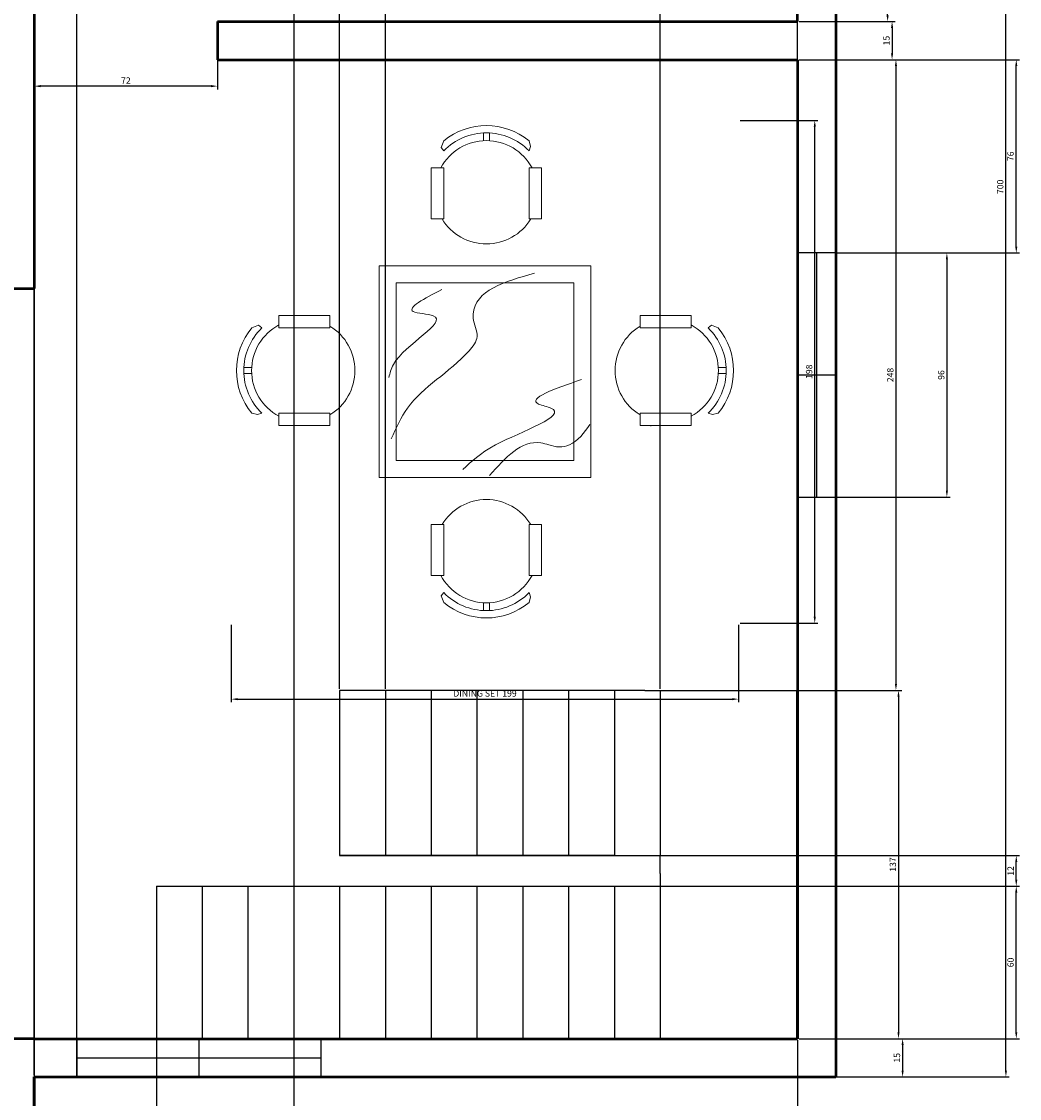
# Model space of a CAD drawing. Units: inches. Extents: x 604 to 3492, y -123 to 1737.
# Tile 9 of 20: x 1033 to 1425, y 579 to 1003. Entities that reach past the tile are written whole.
import ezdxf

# ---------------------------------------------------------------- set-up
doc = ezdxf.new("R2010")
doc.units = ezdxf.units.IN
for name, color, linetype, lineweight in [('A-ANNO-DIMS', 2, 'Continuous', 18), ('A-FLOR-STRS', 7, 'Continuous', 25), ('A-FURN', 8, 'Continuous', 18), ('A-GLAZ', 4, 'Continuous', 25), ('A-WALL', 7, 'Continuous', 50)]:
    doc.layers.add(name, color=color, linetype=linetype, lineweight=lineweight)
doc.styles.get("Standard").update_dxf_attribs({"font": 'arial.ttf'})
doc.dimstyles.new('ISO-25', dxfattribs={"dimtxt": 2.5, "dimasz": 2.5, "dimexe": 1.25, "dimexo": 0.625, "dimtad": 1, "dimtxsty": 'Standard', "dimcen": 2.5, "dimadec": 0, "dimazin": 0, "dimtfac": 1, "dimtmove": 0, "dimatfit": 3, "dimfxl": 1, "dimarcsym": 0})

# ---------------------------------------------------------------- blocks, each defined once
blk = doc.blocks.new('A$C654B463E')
for p, q in [((1.0495, 2.0294), (1.0495, 2.0624)), ((1.0746, 2.0294), (1.0746, 2.0624)), ((0.8807, 2.0283), (0.8697, 2.0004)), ((1.249, 2.0041), (1.2435, 2.0283)), ((0.8697, 2.0004), (0.8807, 1.9859)), ((1.2435, 1.9859), (1.249, 2.0041)), ((0.828, 1.9133), (0.828, 1.6966)), ((0.8808, 1.9133), (0.828, 1.9133)), ((0.8808, 1.6966), (0.8808, 1.9133)), ((1.2433, 1.6966), (1.2433, 1.9133)), ((1.2433, 1.9133), (1.2962, 1.9133)), ((1.2962, 1.9133), (1.2962, 1.6966)), ((0.828, 1.6966), (0.8808, 1.6966)), ((1.2962, 1.6966), (1.2433, 1.6966)), ((1.5061, 1.4969), (0.6061, 1.4969)), ((0.6061, 1.4969), (0.6061, 0.5969)), ((1.5061, 0.5969), (1.5061, 1.4969)), ((1.4341, 1.4249), (0.6781, 1.4249)), ((0.6781, 1.4249), (0.6781, 0.6689)), ((1.4341, 0.6689), (1.4341, 1.4249)), ((0.1805, 1.2861), (0.3972, 1.2861)), ((0.1805, 1.2332), (0.1805, 1.2861)), ((0.3972, 1.2861), (0.3972, 1.2332)), ((1.9318, 1.2861), (1.7151, 1.2861)), ((1.7151, 1.2861), (1.7151, 1.2332)), ((1.9318, 1.2332), (1.9318, 1.2861)), ((0.0655, 1.2333), (0.0934, 1.2443)), ((0.0934, 1.2443), (0.1079, 1.2333)), ((2.0189, 1.2443), (2.0044, 1.2333)), ((2.0467, 1.2333), (2.0189, 1.2443)), ((0.3972, 1.2332), (0.1805, 1.2332)), ((1.7151, 1.2332), (1.9318, 1.2332)), ((0.0644, 1.0645), (0.0314, 1.0645)), ((2.0478, 1.0645), (2.0808, 1.0645)), ((0.0644, 1.0394), (0.0314, 1.0394)), ((2.0478, 1.0394), (2.0808, 1.0394)), ((0.0897, 0.8651), (0.0655, 0.8706)), ((0.1079, 0.8706), (0.0897, 0.8651)), ((0.3972, 0.8707), (0.1805, 0.8707)), ((0.1805, 0.8707), (0.1805, 0.8178)), ((0.3972, 0.8178), (0.3972, 0.8707)), ((1.7151, 0.8178), (1.7151, 0.8707)), ((1.7151, 0.8707), (1.9318, 0.8707)), ((1.9318, 0.8707), (1.9318, 0.8178)), ((2.0044, 0.8706), (2.0226, 0.8651)), ((2.0226, 0.8651), (2.0467, 0.8706)), ((0.1805, 0.8178), (0.3972, 0.8178)), ((1.9318, 0.8178), (1.7151, 0.8178)), ((1.7602, 0.816), (1.7602, 0.8178)), ((0.6781, 0.6689), (1.4341, 0.6689)), ((0.6061, 0.5969), (1.5061, 0.5969)), ((0.828, 0.1805), (0.828, 0.3972)), ((0.828, 0.3972), (0.8808, 0.3972)), ((0.8808, 0.3972), (0.8808, 0.1805)), ((1.2962, 0.3972), (1.2433, 0.3972)), ((1.2433, 0.3972), (1.2433, 0.1805)), ((1.2962, 0.1805), (1.2962, 0.3972)), ((0.8808, 0.1805), (0.828, 0.1805)), ((1.2433, 0.1805), (1.2962, 0.1805)), ((0.8697, 0.0934), (0.8807, 0.1079)), ((0.8807, 0.0655), (0.8697, 0.0934)), ((1.2435, 0.1079), (1.249, 0.0897)), ((1.0495, 0.0644), (1.0495, 0.0314)), ((1.0746, 0.0644), (1.0746, 0.0314)), ((1.249, 0.0897), (1.2435, 0.0655))]:
    blk.add_line(p, q)
for centre, radius, start, end in [((1.0621, 1.81), 0.2838, 50.2727, 129.7273), ((1.0621, 1.81), 0.2527, 44.1212, 135.8788), ((1.0621, 1.81), 0.2197, 28.0535, 151.9465), ((1.0621, 1.81), 0.2197, 211.0762, 328.9238), ((0.2838, 1.0519), 0.2197, 118.0535, 241.9465), ((0.2838, 1.0519), 0.2197, 301.0762, 58.9238), ((1.8285, 1.0519), 0.2197, 121.0762, 238.9238), ((1.8285, 1.0519), 0.2197, 298.0535, 61.9465), ((0.2838, 1.0519), 0.2838, 140.2727, 219.7273), ((0.2838, 1.0519), 0.2527, 134.1212, 225.8788), ((1.8285, 1.0519), 0.2527, 314.1212, 45.8788), ((1.8285, 1.0519), 0.2838, 320.2727, 39.7273), ((1.0621, 0.2838), 0.2197, 31.0762, 148.9238), ((1.0621, 0.2838), 0.2197, 208.0535, 331.9465), ((1.0621, 0.2838), 0.2527, 224.1212, 315.8788), ((1.0621, 0.2838), 0.2838, 230.2727, 309.7273)]:
    blk.add_arc(centre, radius, start, end)
for points, knots in [([(1.2668, 1.4661), (1.1404, 1.4303), (1.007, 1.3925), (1.0046, 1.2536), (1.0397, 1.1982), (0.9231, 1.0507), (0.7498, 0.9639), (0.6784, 0.8076), (0.6575, 0.7619)], [0, 0, 0, 0, 0.3137239, 0.3311142, 0.4112811, 0.4813998, 0.8384073, 0.9862554, 0.9862554, 0.9862554, 0.9862554]), ([(0.8733, 1.3971), (0.7986, 1.3581), (0.6818, 1.297), (0.9617, 1.2888), (0.674, 1.1429), (0.652, 1.0406), (0.648, 1.022)], [0, 0, 0, 0, 0.1539075, 0.2404518, 0.5071296, 0.5664465, 0.5664465, 0.5664465, 0.5664465]), ([(1.4669, 1.014), (1.3503, 0.9736), (1.2031, 0.9226), (1.4485, 0.8729), (1.0905, 0.7545), (0.9976, 0.6654), (0.9621, 0.6314)], [0, 0, 0, 0, 0.2104664, 0.2655089, 0.5478612, 0.7218742, 0.7218742, 0.7218742, 0.7218742]), ([(1.0753, 0.6053), (1.1429, 0.6813), (1.22, 0.7679), (1.3305, 0.7349), (1.3708, 0.7234), (1.4433, 0.7391), (1.477, 0.7873), (1.5018, 0.8227)], [0, 0, 0, 0, 0.2582689, 0.2941543, 0.338534, 0.3829138, 0.5059421, 0.5059421, 0.5059421, 0.5059421])]:
    blk.add_open_spline(points, degree=3, knots=knots)
blk = doc.blocks.new('*D15')
at = {"layer": 'A-ANNO-DIMS', "color": 0, "lineweight": -2, "transparency": 16777216}
for p, q in [((1338.64, 1272.7), (1374.65, 1272.7)), ((1373.4, 1005.2), (1373.4, 1270.2)), ((1338.64, 1002.7), (1374.65, 1002.7))]:
    blk.add_line(p, q, dxfattribs=at)
at = {"layer": 'A-ANNO-DIMS', "color": 0, "transparency": 16777216}
for points in [[(1372.98, 1270.2), (1373.81, 1270.2), (1373.4, 1272.7)], [(1372.98, 1005.2), (1373.81, 1005.2), (1373.4, 1002.7)]]:
    blk.add_solid(points, dxfattribs=at)
at = {"layer": 'Defpoints', "color": 0, "transparency": 16777216}
for p in [(1338.01, 1272.7), (1373.4, 1272.7), (1338.01, 1002.7)]:
    blk.add_point(p, dxfattribs=at)
at = {"layer": 'A-ANNO-DIMS', "color": 0, "transparency": 16777216, "insert": (1371.49, 1137.7), "char_height": 2.5, "attachment_point": 5, "rotation": 90}
blk.add_mtext('270', dxfattribs=at)
blk = doc.blocks.new('*D16')
at = {"layer": 'A-ANNO-DIMS', "color": 0, "lineweight": -2, "transparency": 16777216}
for p, q in [((1338.64, 1002.7), (1376.4, 1002.7)), ((1375.15, 1000.2), (1375.15, 990.2)), ((1338.64, 987.7), (1376.4, 987.7))]:
    blk.add_line(p, q, dxfattribs=at)
at = {"layer": 'A-ANNO-DIMS', "color": 0, "transparency": 16777216}
for points in [[(1374.73, 1000.2), (1375.57, 1000.2), (1375.15, 1002.7)], [(1374.73, 990.2), (1375.57, 990.2), (1375.15, 987.7)]]:
    blk.add_solid(points, dxfattribs=at)
at = {"layer": 'Defpoints', "color": 0, "transparency": 16777216}
for p in [(1338.01, 1002.7), (1338.01, 987.7), (1375.15, 987.7)]:
    blk.add_point(p, dxfattribs=at)
at = {"layer": 'A-ANNO-DIMS', "color": 0, "transparency": 16777216, "insert": (1373.25, 995.2), "char_height": 2.5, "attachment_point": 5, "rotation": 90}
blk.add_mtext('15', dxfattribs=at)
blk = doc.blocks.new('*D17')
at = {"layer": 'A-ANNO-DIMS', "color": 0, "lineweight": -2, "transparency": 16777216}
for p, q in [((1338.64, 987.7), (1377.92, 987.7)), ((1376.67, 985.2), (1376.67, 742.2)), ((1338.64, 739.7), (1377.92, 739.7))]:
    blk.add_line(p, q, dxfattribs=at)
at = {"layer": 'A-ANNO-DIMS', "color": 0, "transparency": 16777216}
for points in [[(1376.25, 985.2), (1377.09, 985.2), (1376.67, 987.7)], [(1376.25, 742.2), (1377.09, 742.2), (1376.67, 739.7)]]:
    blk.add_solid(points, dxfattribs=at)
at = {"layer": 'Defpoints', "color": 0, "transparency": 16777216}
for p in [(1338.01, 987.7), (1338.01, 739.7), (1376.67, 739.7)]:
    blk.add_point(p, dxfattribs=at)
at = {"layer": 'A-ANNO-DIMS', "color": 0, "transparency": 16777216, "insert": (1374.77, 863.7), "char_height": 2.5, "attachment_point": 5, "rotation": 90}
blk.add_mtext('248', dxfattribs=at)
blk = doc.blocks.new('*D18')
at = {"layer": 'A-ANNO-DIMS', "color": 0, "lineweight": -2, "transparency": 16777216}
for p, q in [((1338.64, 739.7), (1378.92, 739.7)), ((1377.67, 737.2), (1377.67, 605.2)), ((1338.64, 602.7), (1378.92, 602.7))]:
    blk.add_line(p, q, dxfattribs=at)
at = {"layer": 'A-ANNO-DIMS', "color": 0, "transparency": 16777216}
for points in [[(1377.26, 737.2), (1378.09, 737.2), (1377.67, 739.7)], [(1377.26, 605.2), (1378.09, 605.2), (1377.67, 602.7)]]:
    blk.add_solid(points, dxfattribs=at)
at = {"layer": 'Defpoints', "color": 0, "transparency": 16777216}
for p in [(1338.01, 739.7), (1338.01, 602.7), (1377.67, 602.7)]:
    blk.add_point(p, dxfattribs=at)
at = {"layer": 'A-ANNO-DIMS', "color": 0, "transparency": 16777216, "insert": (1375.77, 671.2), "char_height": 2.5, "attachment_point": 5, "rotation": 90}
blk.add_mtext('137', dxfattribs=at)
blk = doc.blocks.new('*D19')
at = {"layer": 'A-ANNO-DIMS', "color": 0, "lineweight": -2, "transparency": 16777216}
for p, q in [((1338.64, 602.7), (1380.54, 602.7)), ((1379.29, 600.2), (1379.29, 590.2)), ((1338.64, 587.7), (1380.54, 587.7))]:
    blk.add_line(p, q, dxfattribs=at)
at = {"layer": 'A-ANNO-DIMS', "color": 0, "transparency": 16777216}
for points in [[(1378.87, 600.2), (1379.71, 600.2), (1379.29, 602.7)], [(1378.87, 590.2), (1379.71, 590.2), (1379.29, 587.7)]]:
    blk.add_solid(points, dxfattribs=at)
at = {"layer": 'Defpoints', "color": 0, "transparency": 16777216}
for p in [(1338.01, 602.7), (1338.01, 587.7), (1379.29, 587.7)]:
    blk.add_point(p, dxfattribs=at)
at = {"layer": 'A-ANNO-DIMS', "color": 0, "transparency": 16777216, "insert": (1377.39, 595.2), "char_height": 2.5, "attachment_point": 5, "rotation": 90}
blk.add_mtext('15', dxfattribs=at)
blk = doc.blocks.new('*D20')
at = {"layer": 'A-ANNO-DIMS', "color": 0, "lineweight": -2, "transparency": 16777216}
for p, q in [((1353.64, 1287.7), (1421.14, 1287.7)), ((1419.89, 590.2), (1419.89, 1285.2)), ((1353.64, 587.7), (1421.14, 587.7))]:
    blk.add_line(p, q, dxfattribs=at)
at = {"layer": 'A-ANNO-DIMS', "color": 0, "transparency": 16777216}
for points in [[(1419.47, 1285.2), (1420.3, 1285.2), (1419.89, 1287.7)], [(1419.47, 590.2), (1420.3, 590.2), (1419.89, 587.7)]]:
    blk.add_solid(points, dxfattribs=at)
at = {"layer": 'Defpoints', "color": 0, "transparency": 16777216}
for p in [(1353.01, 1287.7), (1419.89, 1287.7), (1353.01, 587.7)]:
    blk.add_point(p, dxfattribs=at)
at = {"layer": 'A-ANNO-DIMS', "color": 0, "transparency": 16777216, "insert": (1417.98, 937.7), "char_height": 2.5, "attachment_point": 5, "rotation": 90}
blk.add_mtext('700', dxfattribs=at)
blk = doc.blocks.new('*D33')
at = {"layer": 'A-ANNO-DIMS', "color": 0, "lineweight": -2, "transparency": 16777216}
for p, q in [((1038.01, 1002.08), (1038.01, 976.04)), ((1110.01, 1002.08), (1110.01, 976.04)), ((1107.51, 977.29), (1040.51, 977.29))]:
    blk.add_line(p, q, dxfattribs=at)
at = {"layer": 'A-ANNO-DIMS', "color": 0, "transparency": 16777216}
for points in [[(1040.51, 977.71), (1040.51, 976.88), (1038.01, 977.29)], [(1107.51, 977.71), (1107.51, 976.88), (1110.01, 977.29)]]:
    blk.add_solid(points, dxfattribs=at)
at = {"layer": 'Defpoints', "color": 0, "transparency": 16777216}
for p in [(1038.01, 1002.7), (1110.01, 1002.7), (1038.01, 977.29)]:
    blk.add_point(p, dxfattribs=at)
at = {"layer": 'A-ANNO-DIMS', "color": 0, "transparency": 16777216, "insert": (1074.01, 979.17), "char_height": 2.5, "attachment_point": 5}
blk.add_mtext('72', dxfattribs=at)
blk = doc.blocks.new('*D34')
at = {"layer": 'A-ANNO-DIMS', "color": 0, "lineweight": -2, "transparency": 16777216}
for p, q in [((1353.64, 911.7), (1397.94, 911.7)), ((1396.69, 909.2), (1396.69, 818.2)), ((1353.64, 815.7), (1397.94, 815.7))]:
    blk.add_line(p, q, dxfattribs=at)
at = {"layer": 'A-ANNO-DIMS', "color": 0, "transparency": 16777216}
for points in [[(1396.28, 909.2), (1397.11, 909.2), (1396.69, 911.7)], [(1396.28, 818.2), (1397.11, 818.2), (1396.69, 815.7)]]:
    blk.add_solid(points, dxfattribs=at)
at = {"layer": 'Defpoints', "color": 0, "transparency": 16777216}
for p in [(1353.01, 911.7), (1353.01, 815.7), (1396.69, 815.7)]:
    blk.add_point(p, dxfattribs=at)
at = {"layer": 'A-ANNO-DIMS', "color": 0, "transparency": 16777216, "insert": (1394.79, 863.7), "char_height": 2.5, "attachment_point": 5, "rotation": 90}
blk.add_mtext('96', dxfattribs=at)
blk = doc.blocks.new('WIN-96')
for p, q in [((15, 96), (0, 96)), ((7.5, 96), (7.5, 0)), ((15, 96), (15, 0)), ((15, 48), (0, 48))]:
    blk.add_line(p, q)
blk.add_lwpolyline([(0, 96), (0, 0), (15, 0), (15, 96)], close=True)
blk = doc.blocks.new('*D83')
at = {"layer": 'A-ANNO-DIMS', "color": 0, "lineweight": -2, "transparency": 16777216}
for p, q in [((1115.46, 765.52), (1115.46, 734.99)), ((1314.85, 765.52), (1314.85, 734.99)), ((1117.96, 736.24), (1312.35, 736.24))]:
    blk.add_line(p, q, dxfattribs=at)
at = {"layer": 'A-ANNO-DIMS', "color": 0, "transparency": 16777216}
for points in [[(1117.96, 736.65), (1117.96, 735.82), (1115.46, 736.24)], [(1312.35, 736.65), (1312.35, 735.82), (1314.85, 736.24)]]:
    blk.add_solid(points, dxfattribs=at)
at = {"layer": 'Defpoints', "color": 0, "transparency": 16777216}
for p in [(1115.46, 766.14), (1314.85, 766.14), (1314.85, 736.24)]:
    blk.add_point(p, dxfattribs=at)
at = {"layer": 'A-ANNO-DIMS', "color": 0, "transparency": 16777216, "insert": (1215.16, 738.15), "char_height": 2.5, "attachment_point": 5}
blk.add_mtext('DINING SET 199', dxfattribs=at)
blk = doc.blocks.new('*D84')
at = {"layer": 'A-ANNO-DIMS', "color": 0, "lineweight": -2, "transparency": 16777216}
for p, q in [((1315.48, 963.83), (1346.01, 963.83)), ((1344.76, 768.64), (1344.76, 961.33)), ((1315.48, 766.14), (1346.01, 766.14))]:
    blk.add_line(p, q, dxfattribs=at)
at = {"layer": 'A-ANNO-DIMS', "color": 0, "transparency": 16777216}
for points in [[(1344.34, 961.33), (1345.18, 961.33), (1344.76, 963.83)], [(1344.34, 768.64), (1345.18, 768.64), (1344.76, 766.14)]]:
    blk.add_solid(points, dxfattribs=at)
at = {"layer": 'Defpoints', "color": 0, "transparency": 16777216}
for p in [(1314.85, 963.83), (1344.76, 963.83), (1314.85, 766.14)]:
    blk.add_point(p, dxfattribs=at)
at = {"layer": 'A-ANNO-DIMS', "color": 0, "transparency": 16777216, "insert": (1342.86, 864.99), "char_height": 2.5, "attachment_point": 5, "rotation": 90}
blk.add_mtext('198', dxfattribs=at)
blk = doc.blocks.new('*D86')
at = {"layer": 'A-ANNO-DIMS', "color": 0, "lineweight": -2, "transparency": 16777216}
for p, q in [((1038.01, 1272.08), (1038.01, 67.77)), ((1140.01, 1272.08), (1140.01, 67.77)), ((1040.51, 69.02), (1137.51, 69.02))]:
    blk.add_line(p, q, dxfattribs=at)
at = {"layer": 'A-ANNO-DIMS', "color": 0, "transparency": 16777216}
for points in [[(1040.51, 69.44), (1040.51, 68.61), (1038.01, 69.02)], [(1137.51, 69.44), (1137.51, 68.61), (1140.01, 69.02)]]:
    blk.add_solid(points, dxfattribs=at)
at = {"layer": 'Defpoints', "color": 0, "transparency": 16777216}
for p in [(1038.01, 1272.7), (1140.01, 1272.7), (1140.01, 69.02)]:
    blk.add_point(p, dxfattribs=at)
at = {"layer": 'A-ANNO-DIMS', "color": 0, "transparency": 16777216, "insert": (1089.01, 70.93), "char_height": 2.5, "attachment_point": 5}
blk.add_mtext('102', dxfattribs=at)
blk = doc.blocks.new('*D88')
at = {"layer": 'A-ANNO-DIMS', "color": 0, "lineweight": -2, "transparency": 16777216}
for p, q in [((1338.64, 987.7), (1425.21, 987.7)), ((1423.96, 914.2), (1423.96, 985.2)), ((1353.64, 911.7), (1425.21, 911.7))]:
    blk.add_line(p, q, dxfattribs=at)
at = {"layer": 'A-ANNO-DIMS', "color": 0, "transparency": 16777216}
for points in [[(1423.54, 985.2), (1424.38, 985.2), (1423.96, 987.7)], [(1423.54, 914.2), (1424.38, 914.2), (1423.96, 911.7)]]:
    blk.add_solid(points, dxfattribs=at)
at = {"layer": 'Defpoints', "color": 0, "transparency": 16777216}
for p in [(1338.01, 987.7), (1423.96, 987.7), (1353.01, 911.7)]:
    blk.add_point(p, dxfattribs=at)
at = {"layer": 'A-ANNO-DIMS', "color": 0, "transparency": 16777216, "insert": (1422.06, 949.7), "char_height": 2.5, "attachment_point": 5, "rotation": 90}
blk.add_mtext('76', dxfattribs=at)
blk = doc.blocks.new('*D93')
at = {"layer": 'A-ANNO-DIMS', "color": 0, "lineweight": -2, "transparency": 16777216}
for p, q in [((1038.01, 588.33), (1038.01, 1359.9)), ((1054.71, 588.27), (1054.71, 1359.9)), ((1040.51, 1358.65), (1052.21, 1358.65))]:
    blk.add_line(p, q, dxfattribs=at)
at = {"layer": 'A-ANNO-DIMS', "color": 0, "transparency": 16777216}
for points in [[(1040.51, 1359.07), (1040.51, 1358.23), (1038.01, 1358.65)], [(1052.21, 1359.07), (1052.21, 1358.23), (1054.71, 1358.65)]]:
    blk.add_solid(points, dxfattribs=at)
at = {"layer": 'Defpoints', "color": 0, "transparency": 16777216}
for p in [(1054.71, 1358.65), (1038.01, 587.7), (1054.71, 587.64)]:
    blk.add_point(p, dxfattribs=at)
at = {"layer": 'A-ANNO-DIMS', "color": 0, "transparency": 16777216, "insert": (1046.36, 1360.55), "char_height": 2.5, "attachment_point": 5}
blk.add_mtext('16.697', dxfattribs=at)
blk = doc.blocks.new('*D94')
at = {"layer": 'A-ANNO-DIMS', "color": 0, "lineweight": -2, "transparency": 16777216}
for p, q in [((1086.01, 602.08), (1086.01, 67.77)), ((1338.01, 602.08), (1338.01, 67.77)), ((1088.51, 69.02), (1335.51, 69.02))]:
    blk.add_line(p, q, dxfattribs=at)
at = {"layer": 'A-ANNO-DIMS', "color": 0, "transparency": 16777216}
for points in [[(1088.51, 69.44), (1088.51, 68.61), (1086.01, 69.02)], [(1335.51, 69.44), (1335.51, 68.61), (1338.01, 69.02)]]:
    blk.add_solid(points, dxfattribs=at)
at = {"layer": 'Defpoints', "color": 0, "transparency": 16777216}
for p in [(1086.01, 602.7), (1338.01, 602.7), (1338.01, 69.02)]:
    blk.add_point(p, dxfattribs=at)
at = {"layer": 'A-ANNO-DIMS', "color": 0, "transparency": 16777216, "insert": (1212.01, 70.93), "char_height": 2.5, "attachment_point": 5}
blk.add_mtext('252', dxfattribs=at)
blk = doc.blocks.new('*D95')
at = {"layer": 'A-ANNO-DIMS', "color": 0, "lineweight": -2, "transparency": 16777216}
for p, q in [((1284.01, 740.33), (1284.01, 1359.9)), ((1338.01, 740.33), (1338.01, 1359.9)), ((1286.51, 1358.65), (1335.51, 1358.65))]:
    blk.add_line(p, q, dxfattribs=at)
at = {"layer": 'A-ANNO-DIMS', "color": 0, "transparency": 16777216}
for points in [[(1286.51, 1359.07), (1286.51, 1358.23), (1284.01, 1358.65)], [(1335.51, 1359.07), (1335.51, 1358.23), (1338.01, 1358.65)]]:
    blk.add_solid(points, dxfattribs=at)
at = {"layer": 'Defpoints', "color": 0, "transparency": 16777216}
for p in [(1338.01, 1358.65), (1284.01, 739.7), (1338.01, 739.7)]:
    blk.add_point(p, dxfattribs=at)
at = {"layer": 'A-ANNO-DIMS', "color": 0, "transparency": 16777216, "insert": (1311.01, 1360.55), "char_height": 2.5, "attachment_point": 5}
blk.add_mtext('54', dxfattribs=at)
blk = doc.blocks.new('*D96')
at = {"layer": 'A-ANNO-DIMS', "color": 0, "lineweight": -2, "transparency": 16777216}
for p, q in [((1158.01, 740.33), (1158.01, 1359.9)), ((1176.01, 740.33), (1176.01, 1359.9)), ((1160.51, 1358.65), (1173.51, 1358.65))]:
    blk.add_line(p, q, dxfattribs=at)
at = {"layer": 'A-ANNO-DIMS', "color": 0, "transparency": 16777216}
for points in [[(1160.51, 1359.07), (1160.51, 1358.23), (1158.01, 1358.65)], [(1173.51, 1359.07), (1173.51, 1358.23), (1176.01, 1358.65)]]:
    blk.add_solid(points, dxfattribs=at)
at = {"layer": 'Defpoints', "color": 0, "transparency": 16777216}
for p in [(1176.01, 1358.65), (1158.01, 739.7), (1176.01, 739.7)]:
    blk.add_point(p, dxfattribs=at)
at = {"layer": 'A-ANNO-DIMS', "color": 0, "transparency": 16777216, "insert": (1167.01, 1360.55), "char_height": 2.5, "attachment_point": 5}
blk.add_mtext('18', dxfattribs=at)
blk = doc.blocks.new('*D97')
at = {"layer": 'A-ANNO-DIMS', "color": 0, "lineweight": -2, "transparency": 16777216}
for p, q in [((1338.64, 662.7), (1425.21, 662.7)), ((1423.96, 605.2), (1423.96, 660.2)), ((1338.64, 602.7), (1425.21, 602.7))]:
    blk.add_line(p, q, dxfattribs=at)
at = {"layer": 'A-ANNO-DIMS', "color": 0, "transparency": 16777216}
for points in [[(1423.54, 660.2), (1424.38, 660.2), (1423.96, 662.7)], [(1423.54, 605.2), (1424.38, 605.2), (1423.96, 602.7)]]:
    blk.add_solid(points, dxfattribs=at)
at = {"layer": 'Defpoints', "color": 0, "transparency": 16777216}
for p in [(1338.01, 662.7), (1423.96, 662.7), (1338.01, 602.7)]:
    blk.add_point(p, dxfattribs=at)
at = {"layer": 'A-ANNO-DIMS', "color": 0, "transparency": 16777216, "insert": (1422.06, 632.7), "char_height": 2.5, "attachment_point": 5, "rotation": 90}
blk.add_mtext('60', dxfattribs=at)
blk = doc.blocks.new('*D98')
at = {"layer": 'A-ANNO-DIMS', "color": 0, "lineweight": -2, "transparency": 16777216}
for p, q in [((1338.64, 674.7), (1425.21, 674.7)), ((1423.96, 665.2), (1423.96, 672.2)), ((1338.64, 662.7), (1425.21, 662.7))]:
    blk.add_line(p, q, dxfattribs=at)
at = {"layer": 'A-ANNO-DIMS', "color": 0, "transparency": 16777216}
for points in [[(1423.54, 672.2), (1424.38, 672.2), (1423.96, 674.7)], [(1423.54, 665.2), (1424.38, 665.2), (1423.96, 662.7)]]:
    blk.add_solid(points, dxfattribs=at)
at = {"layer": 'Defpoints', "color": 0, "transparency": 16777216}
for p in [(1338.01, 674.7), (1423.96, 674.7), (1338.01, 662.7)]:
    blk.add_point(p, dxfattribs=at)
at = {"layer": 'A-ANNO-DIMS', "color": 0, "transparency": 16777216, "insert": (1422.08, 668.7), "char_height": 2.5, "attachment_point": 5, "rotation": 90}
blk.add_mtext('12', dxfattribs=at)

msp = doc.modelspace()

# ---------------------------------------------------------------- linework, layer by layer
at = {"layer": 'A-FLOR-STRS'}
for p, q in [((1158.0111, 739.7004), (1158.0111, 674.7004)), ((1176.0111, 739.7004), (1176.0111, 674.7004)), ((1176.0111, 739.7004), (1176.0111, 674.7004)), ((1194.0111, 739.7004), (1194.0111, 674.7004)), ((1194.0111, 739.7004), (1194.0111, 674.7004)), ((1212.0111, 739.7004), (1212.0111, 674.7004)), ((1212.0111, 739.7004), (1212.0111, 674.7004)), ((1230.0111, 739.7004), (1230.0111, 674.7004)), ((1230.0111, 739.7004), (1230.0111, 674.7004)), ((1248.0111, 739.7004), (1248.0111, 674.7004)), ((1248.0111, 739.7004), (1248.0111, 674.7004)), ((1266.0111, 739.7004), (1266.0111, 674.7004)), ((1266.0111, 739.7004), (1266.0111, 674.7004)), ((1278.0111, 739.7004), (1338.0111, 739.7004)), ((1284.0111, 739.7004), (1284.0111, 674.7004)), ((1266.0111, 674.7004), (1158.0111, 674.7004)), ((1266.0111, 674.7004), (1284.0111, 674.7004)), ((1284.0111, 667.7004), (1284.0111, 674.7004)), ((1284.0111, 674.7004), (1338.0111, 674.7004)), ((1284.0111, 667.7004), (1284.0111, 602.7004)), ((1086.0111, 662.7004), (1266.0111, 662.7004)), ((1086.0111, 662.7004), (1086.0111, 602.7004)), ((1104.0111, 662.7004), (1104.0111, 602.7004)), ((1122.0111, 662.7004), (1122.0111, 602.7004)), ((1122.0111, 662.7004), (1122.0111, 602.7004)), ((1140.0111, 662.7004), (1140.0111, 602.7004)), ((1158.0111, 662.7004), (1158.0111, 602.7004)), ((1176.0111, 662.7004), (1176.0111, 602.7004)), ((1194.0111, 662.7004), (1194.0111, 602.7004)), ((1194.0111, 662.7004), (1194.0111, 602.7004)), ((1212.0111, 662.7004), (1212.0111, 602.7004)), ((1230.0111, 662.7004), (1230.0111, 602.7004)), ((1248.0111, 662.7004), (1248.0111, 602.7004)), ((1266.0111, 662.7004), (1266.0111, 602.7004)), ((1266.0111, 662.7004), (1266.0111, 602.7004)), ((1266.0111, 662.7004), (1284.0111, 662.7004)), ((1284.0111, 662.7004), (1338.0111, 662.7004))]:
    msp.add_line(p, q, dxfattribs=at)
msp.add_lwpolyline([(1278.0111, 739.7004), (1158.0111, 739.7004), (1158.0111, 674.7004), (1266.0111, 674.7004)], dxfattribs=at)
at = {"layer": 'A-WALL'}
for p, q in [((1353.0111, 1287.7004), (1353.0111, 587.7004)), ((1038.0111, 1272.7004), (1038.0111, 897.7004)), ((1338.0111, 1002.7004), (1338.0111, 1272.7004)), ((1038.0111, 1002.7004), (1038.0111, 987.7004)), ((1110.0111, 1002.7004), (1338.0111, 1002.7004)), ((1110.0111, 1002.7004), (1110.0111, 987.7004)), ((1110.0111, 987.7004), (1338.0111, 987.7004)), ((1338.0111, 987.7004), (1338.0111, 602.7004)), ((1338.0111, 987.7004), (1338.0111, 739.7004)), ((1017.0111, 897.7004), (1038.0111, 897.7004)), ((1338.0111, 602.7004), (1338.0111, 739.7004)), ((1038.0111, 602.7004), (1338.0111, 602.7004)), ((1038.0111, 587.7004), (1338.0111, 587.7004)), ((1038.0111, 587.7004), (1038.0111, 287.7004)), ((1338.0111, 587.7004), (1353.0111, 587.7004))]:
    msp.add_line(p, q, dxfattribs=at)
for points in [[(1038.0111, 602.7004), (1023.0111, 602.7004), (1023.0111, 422.7004)], [(1038.0111, 422.7004), (1038.0111, 587.7004)]]:
    msp.add_lwpolyline(points, dxfattribs=at)

# ---------------------------------------------------------------- block references
at = {"layer": 'A-FURN', "xscale": 92.48367459558828, "yscale": 92.48367459558828, "zscale": 92.48367459558828}
msp.add_blockref('A$C654B463E', (1117.4814, 768.1642), dxfattribs=at)
at = {"layer": 'A-GLAZ'}
msp.add_blockref('WIN-96', (1338.0111, 815.7004), dxfattribs=at)
at = {"layer": 'A-GLAZ', "rotation": 89.99999999999982}
msp.add_blockref('WIN-96', (1150.7083, 587.6435), dxfattribs=at)

# ---------------------------------------------------------------- dimensions: what is measured, and where the dimension line sits
at = {"layer": 'A-ANNO-DIMS'}
for base, p1, p2, override, picture, middle in [((1054.7083, 1358.6504), (1038.0111, 587.7004), (1054.7083, 587.6435), {"dimdec": 3, "dimlfac": 1, "dimrnd": 0, "dimzin": 0, "dimdsep": 46, "dimlunit": 2}, '*D93', (1046.3597, 1360.5519)), ((1176.0111, 1358.6504), (1158.0111, 739.7004), (1176.0111, 739.7004), {"dimdec": 0, "dimlfac": 1, "dimrnd": 0, "dimzin": 0, "dimdsep": 46, "dimlunit": 2}, '*D96', (1167.0111, 1360.5519)), ((1338.0111, 1358.6504), (1284.0111, 739.7004), (1338.0111, 739.7004), {"dimdec": 0, "dimlfac": 1, "dimrnd": 0, "dimzin": 0, "dimdsep": 46, "dimlunit": 2}, '*D95', (1311.0111, 1360.5468)), ((1140.0111, 69.0242), (1038.0111, 1272.7004), (1140.0111, 1272.7004), {"dimdec": 0, "dimlfac": 1, "dimrnd": 0, "dimzin": 0, "dimdsep": 46, "dimlunit": 2}, '*D86', (1089.0111, 70.9256)), ((1038.0111, 977.2917), (1110.0111, 1002.7004), (1038.0111, 1002.7004), {"dimclrd": 0, "dimclre": 0, "dimclrt": 0}, '*D33', (1074.0111, 979.1718)), ((1338.0111, 69.0242), (1086.0111, 602.7004), (1338.0111, 602.7004), {"dimdec": 0, "dimlfac": 1, "dimrnd": 0, "dimzin": 0, "dimdsep": 46, "dimlunit": 2}, '*D94', (1212.0111, 70.9256))]:
    dim = msp.add_linear_dim(base=base, p1=p1, p2=p2, dimstyle='ISO-25', override=override, dxfattribs=at)
    dim.commit()
    dim.dimension.update_dxf_attribs({"geometry": picture, "text_midpoint": middle})
for base, p1, p2, override, picture, middle in [((1419.8851, 1287.7004), (1353.0111, 587.7004), (1353.0111, 1287.7004), {"dimclrd": 0, "dimclre": 0, "dimclrt": 0}, '*D20', (1417.9836, 937.7004)), ((1375.1487, 987.7004), (1338.0111, 1002.7004), (1338.0111, 987.7004), {"dimclrd": 0, "dimclre": 0, "dimclrt": 0}, '*D16', (1373.2472, 995.2004)), ((1376.6683, 739.7004), (1338.0111, 987.7004), (1338.0111, 739.7004), {"dimclrd": 0, "dimclre": 0, "dimclrt": 0}, '*D17', (1374.7669, 863.7004)), ((1423.9611, 987.7004), (1353.0111, 911.7004), (1338.0111, 987.7004), {"dimdec": 0, "dimlfac": 1, "dimrnd": 0, "dimzin": 0, "dimdsep": 46, "dimlunit": 2}, '*D88', (1422.0597, 949.7004)), ((1344.7607, 963.8263), (1314.8521, 766.1441), (1314.8521, 963.8263), {"dimdec": 0, "dimlfac": 1, "dimrnd": 0, "dimzin": 0, "dimdsep": 46, "dimlunit": 2}, '*D84', (1342.8593, 864.9852)), ((1396.6926, 815.7004), (1353.0111, 911.7004), (1353.0111, 815.7004), {"dimclrd": 0, "dimclre": 0, "dimclrt": 0}, '*D34', (1394.7912, 863.7004)), ((1377.6745, 602.7004), (1338.0111, 739.7004), (1338.0111, 602.7004), {"dimclrd": 0, "dimclre": 0, "dimclrt": 0}, '*D18', (1375.7722, 671.2004)), ((1423.9611, 674.7004), (1338.0111, 662.7004), (1338.0111, 674.7004), {"dimdec": 0, "dimlfac": 1, "dimrnd": 0, "dimzin": 0, "dimdsep": 46, "dimlunit": 2}, '*D98', (1422.081, 668.7004)), ((1423.9611, 662.7004), (1338.0111, 602.7004), (1338.0111, 662.7004), {"dimdec": 0, "dimlfac": 1, "dimrnd": 0, "dimzin": 0, "dimdsep": 46, "dimlunit": 2}, '*D97', (1422.0597, 632.7004))]:
    dim = msp.add_linear_dim(base=base, p1=p1, p2=p2, angle=90, dimstyle='ISO-25', override=override, dxfattribs=at)
    dim.commit()
    dim.dimension.update_dxf_attribs({"geometry": picture, "text_midpoint": middle})
for p1, p2, distance, picture, middle in [((1338.0111, 1002.7004), (1338.0111, 1272.7004), -35.3849, '*D15', (1371.4946, 1137.7004)), ((1338.0111, 602.7004), (1338.0111, 587.7004), 41.2804, '*D19', (1377.3901, 595.2004))]:
    dim = msp.add_aligned_dim(p1=p1, p2=p2, distance=distance, dimstyle='ISO-25', override={"dimclrd": 0, "dimclre": 0, "dimclrt": 0}, dxfattribs=at)
    dim.commit()
    dim.dimension.update_dxf_attribs({"geometry": picture, "text_midpoint": middle})
dim = msp.add_linear_dim(base=(1314.8521, 736.2355), p1=(1115.4612, 766.1441), p2=(1314.8521, 766.1441), text='DINING SET <>', dimstyle='ISO-25', override={"dimdec": 0, "dimlfac": 1, "dimrnd": 0, "dimzin": 0, "dimdsep": 46, "dimlunit": 2}, dxfattribs=at)
dim.commit()
dim.dimension.update_dxf_attribs({"geometry": '*D83', "text_midpoint": (1215.1567, 738.1531)})

doc.saveas('drawing.dxf')
